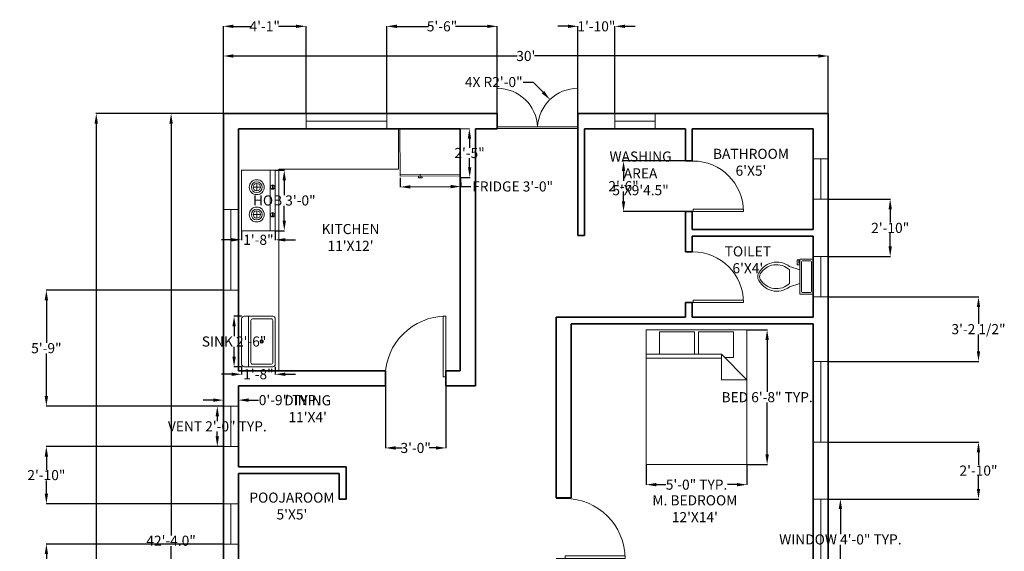
# Model space of a CAD drawing. Units: inches. Extents: x 94 to 277359, y -289541 to 1081.
# Tile 3 of 5: x 94 to 680, y 765 to 1081. Entities that reach past the tile are written whole.
import ezdxf

# ---------------------------------------------------------------- set-up
doc = ezdxf.new("R2010")
doc.units = ezdxf.units.IN
doc.header["$MEASUREMENT"] = 0
doc.layers.get('Defpoints').update_dxf_attribs({"color": 255})
for name, color, linetype, lineweight in [('A-ANNO-DIMS', 2, 'Continuous', 18), ('A-AREA-IDEN', 7, 'Continuous', 18), ('A-DOOR', 4, 'Continuous', 18), ('A-EQPM', 8, 'Continuous', 18), ('A-FLOR-CASE', 8, 'Continuous', 18), ('A-FLOR-FIXT', 8, 'Continuous', 18), ('A-WALL', 7, 'Continuous', 35), ('furniture', 163, 'Continuous', 18), ('window', 13, 'Continuous', 18)]:
    doc.layers.add(name, color=color, linetype=linetype, lineweight=lineweight)
doc.styles.get("Standard").update_dxf_attribs({"font": 'arial.ttf'})
doc.dimstyles.get("Standard").update_dxf_attribs({"dimtxt": 6, "dimasz": 6, "dimexe": 0.18, "dimexo": 0.0625, "dimgap": 0.09, "dimtad": 0, "dimtih": 1, "dimtoh": 1, "dimdec": 1, "dimzin": 0, "dimdsep": 46, "dimlunit": 3, "dimtxsty": 'Standard', "dimcen": 0.09, "dimadec": 0, "dimazin": 0, "dimtfac": 1, "dimtdec": 1, "dimtofl": 0, "dimtmove": 0, "dimatfit": 3, "dimfxl": 1, "dimtolj": 1, "dimtzin": 0, "dimarcsym": 0})

# ---------------------------------------------------------------- blocks, each defined once
blk = doc.blocks.new('DOOR')
for p, q in [((-94.95, 365.26), (-85.95, 365.26)), ((-94.95, 317.26), (-94.95, 365.26)), ((-90.45, 365.26), (-90.45, 317.26)), ((-85.95, 365.26), (-85.95, 317.26)), ((-85.95, 317.26), (-94.95, 317.26))]:
    blk.add_line(p, q)
blk = doc.blocks.new('V')
for p, q in [((-17.52, 401.92), (-8.52, 401.92)), ((-17.52, 377.92), (-17.52, 401.92)), ((-13.02, 377.92), (-13.02, 401.92)), ((-8.52, 401.92), (-8.52, 377.92)), ((-8.52, 377.92), (-17.52, 377.92))]:
    blk.add_line(p, q)
blk = doc.blocks.new('*D3')
at = {"layer": 'A-ANNO-DIMS', "color": 0, "lineweight": -2, "transparency": 16777216}
for p, q in [((215.5, 1025.45), (139.73, 1025.45)), ((139.91, 1019.45), (139.91, 717.61)), ((139.91, 409.45), (139.91, 711.3)), ((215.5, 403.45), (139.73, 403.45))]:
    blk.add_line(p, q, dxfattribs=at)
at = {"layer": 'A-ANNO-DIMS', "color": 0, "transparency": 16777216}
for points in [[(138.91, 1019.45), (140.91, 1019.45), (139.91, 1025.45)], [(138.91, 409.45), (140.91, 409.45), (139.91, 403.45)]]:
    blk.add_solid(points, dxfattribs=at)
at = {"layer": 'Defpoints', "color": 0, "transparency": 16777216}
for p in [(139.91, 1025.45), (215.56, 1025.45), (215.56, 403.45)]:
    blk.add_point(p, dxfattribs=at)
at = {"layer": 'A-ANNO-DIMS', "color": 0, "transparency": 16777216, "insert": (139.91, 714.45), "char_height": 6, "attachment_point": 5}
blk.add_mtext('\\A1;51\'-10.0"', dxfattribs=at)
blk = doc.blocks.new('*D4')
at = {"layer": 'A-ANNO-DIMS', "color": 0, "lineweight": -2, "transparency": 16777216}
for p, q in [((215.5, 1025.45), (184.27, 1025.45)), ((184.45, 1019.45), (184.45, 774.61)), ((184.45, 523.45), (184.45, 768.3)), ((215.5, 517.45), (184.27, 517.45))]:
    blk.add_line(p, q, dxfattribs=at)
at = {"layer": 'A-ANNO-DIMS', "color": 0, "transparency": 16777216}
for points in [[(183.45, 1019.45), (185.45, 1019.45), (184.45, 1025.45)], [(183.45, 523.45), (185.45, 523.45), (184.45, 517.45)]]:
    blk.add_solid(points, dxfattribs=at)
at = {"layer": 'Defpoints', "color": 0, "transparency": 16777216}
for p in [(215.56, 1025.45), (184.45, 517.45), (215.56, 517.45)]:
    blk.add_point(p, dxfattribs=at)
at = {"layer": 'A-ANNO-DIMS', "color": 0, "transparency": 16777216, "insert": (184.45, 771.45), "char_height": 6, "attachment_point": 5}
blk.add_mtext('\\A1;42\'-4.0"', dxfattribs=at)
blk = doc.blocks.new('Bed - Queen')
for p, q in [((0, -80.00003), (0, 0)), ((0, 0), (59.99999, 0)), ((59.99999, 0), (59.99999, -80.00003)), ((7.99999, -1.2), (28.79998, -1.2)), ((7.99999, -14.4), (7.99999, -1.2)), ((28.79998, -1.2), (28.79998, -14.4)), ((31.19999, -1.2), (51.99999, -1.2)), ((31.19999, -14.4), (31.19999, -1.2)), ((51.99999, -1.2), (51.99999, -16.4)), ((0, -14.4), (44.8, -14.4)), ((44.8, -16.8), (0, -16.8)), ((59.99999, -29.6), (44.8, -14.4)), ((44.8, -14.4), (44.8, -29.6)), ((51.99999, -16.4), (46.79936, -16.4)), ((44.8, -29.6), (59.99999, -29.6)), ((59.99999, -80.00003), (0, -80.00003))]:
    blk.add_line(p, q)
blk = doc.blocks.new('Sink-single - 30 in top')
blk.add_line((-15, -3.999996), (15, -3.999996))
for points in [[(-13.5, 0), (13.5, 0)], [(-15, -18.499996), (-15, -1.5)], [(-12.5, -5.499996), (12.5, -5.499996)], [(15, -1.5), (15, -18.499996)], [(-13.5, -17.499996), (-13.5, -6.499996)], [(13.5, -6.499996), (13.5, -17.499996)], [(13.5, -19.999996), (-13.5, -19.999996)], [(12.5, -18.499996), (-12.5, -18.499996)]]:
    blk.add_lwpolyline(points)
for radius in [1, 0.5]:
    blk.add_circle((0, -11.999996), radius)
for centre, radius, start, end in [((-13.5, -1.5), 1.5, 90, 180), ((-12.5, -6.499996), 1, 90, 180), ((12.5, -6.499996), 1, 0, 90), ((13.5, -1.5), 1.5, 0, 90), ((-12.5, -17.499996), 1, 180, 270), ((12.5, -17.499996), 1, 270, 0), ((-13.5, -18.499996), 1.5, 180, 270), ((13.5, -18.499996), 1.5, 270, 0)]:
    blk.add_arc(centre, radius, start, end)
blk = doc.blocks.new('gas')
at = {"layer": 'furniture'}
for p, q in [((194.36, 516.15), (214.36, 516.15)), ((194.36, 480.15), (194.36, 516.15)), ((211.36, 516.15), (211.36, 480.15)), ((214.36, 516.15), (214.36, 480.15)), ((201.2, 506.04), (205.6, 506.04)), ((203.4, 503.83), (203.4, 508.24)), ((212.69, 504.83), (212.69, 507.37)), ((213.08, 504.83), (213.08, 507.37)), ((201.2, 489.79), (205.6, 489.79)), ((203.4, 487.59), (203.4, 492)), ((212.69, 488.4), (212.69, 490.95)), ((213.08, 488.4), (213.08, 490.94)), ((214.36, 480.15), (194.36, 480.15))]:
    blk.add_line(p, q, dxfattribs=at)
for centre, radius in [((203.4, 506.04), 4.44), ((203.4, 506.04), 3.22), ((203.4, 506.04), 2.2), ((212.86, 506.1), 1.29), ((203.4, 489.79), 4.44), ((203.4, 489.79), 3.22), ((203.4, 489.79), 2.2), ((212.86, 489.67), 1.29)]:
    blk.add_circle(centre, radius, dxfattribs=at)
blk = doc.blocks.new('Refrigerator-2 door - 36 in top')
for p, q in [((0, -26.999999), (36, -26.999999)), ((11, -27.999999), (11, -28.999999)), ((11, -28.999999), (13, -28.999999)), ((12, -26.999999), (12, -28.999999)), ((13, -28.999999), (13, -27.999999))]:
    blk.add_line(p, q)
blk.add_lwpolyline([(0, -27.999999), (0, 0), (36, 0), (36, -27.999999)], close=True)
blk = doc.blocks.new('Toilet - top')
for p, q in [((9.5, -6), (9.5, -2)), ((-10, -8.5), (-8, -8.5)), ((-10, -9.5), (-10, -8.5)), ((-7, -9.5), (-10, -9.5)), ((-8, -8.5), (-8, -8)), ((-7, -8), (-7, -9.5)), ((-4, -8), (-6, -14)), ((4, -8), (6, -14)), ((4, -14), (-4, -14))]:
    blk.add_line(p, q)
blk.add_lwpolyline([(10.5, -8), (10.5, 0), (-10.5, 0), (-10.5, -8)], close=True)
for points in [[(-9.5, -2), (-9.5, -6)], [(8.5, -1), (-8.5, -1)], [(-8.5, -7), (8.5, -7)]]:
    blk.add_lwpolyline(points)
for centre, radius, start, end in [((-8.62, -1.88), 0.884, 81.8699, 188.1301), ((8.62, -1.88), 0.884, 351.8699, 98.1301), ((-8.62, -6.12), 0.884, 171.8699, 278.1301), ((8.62, -6.12), 0.884, 261.8699, 8.1301), ((3.52, -21.58), 12.17, 141.46911, 247.97143), ((4.2, -21.82), 11.33, 136.36773, 238.94682), ((-3.52, -21.58), 12.17, 292.02843, 38.53071), ((-4.2, -21.82), 11.33, 301.05301, 43.63209), ((0, -27.88), 4, 245.73182, 294.26817), ((0, -29), 4, 254.86053, 285.13947)]:
    blk.add_arc(centre, radius, start, end)
blk = doc.blocks.new('MD')
for p, q in [((202.8, 674.18), (202.8, 698.18)), ((250.8, 674.18), (250.8, 698.18)), ((202.8, 675.18), (250.8, 675.18)), ((202.8, 674.18), (250.8, 674.18))]:
    blk.add_line(p, q)
for centre, start, end in [((202.8, 674.18), 2.38802, 90), ((250.8, 674.18), 90, 177.61198)]:
    blk.add_arc(centre, 24, start, end)
blk = doc.blocks.new('*U15')
for p, q in [((0, 0), (0, -6)), ((40, 0), (40, -6))]:
    blk.add_line(p, q)
blk.add_lwpolyline([(0, 0), (0, 40), (1.75, 40), (1.75, 0)], close=True)
blk.add_arc((0, 0), 40, 0, 90)
blk = doc.blocks.new('*D16')
at = {"layer": 'A-ANNO-DIMS', "color": 0, "lineweight": -2, "transparency": 16777216}
for p, q in [((215.56, 1025.52), (215.56, 1059.85)), ((221.56, 1059.67), (390.38, 1059.67)), ((569.56, 1059.67), (400.74, 1059.67)), ((575.56, 1025.52), (575.56, 1059.85))]:
    blk.add_line(p, q, dxfattribs=at)
at = {"layer": 'A-ANNO-DIMS', "color": 0, "transparency": 16777216}
for points in [[(221.56, 1060.67), (221.56, 1058.67), (215.56, 1059.67)], [(569.56, 1060.67), (569.56, 1058.67), (575.56, 1059.67)]]:
    blk.add_solid(points, dxfattribs=at)
at = {"layer": 'Defpoints', "color": 0, "transparency": 16777216}
for p in [(575.56, 1059.67), (215.56, 1025.45), (575.56, 1025.45)]:
    blk.add_point(p, dxfattribs=at)
at = {"layer": 'A-ANNO-DIMS', "color": 0, "transparency": 16777216, "insert": (395.56, 1059.67), "char_height": 6, "attachment_point": 5}
blk.add_mtext("\\A1;30'", dxfattribs=at)
blk = doc.blocks.new('*D21')
at = {"layer": 'A-ANNO-DIMS', "color": 0, "lineweight": -2, "transparency": 16777216}
for p, q in [((575.63, 796.21), (582.94, 796.21)), ((582.76, 790.21), (582.76, 775.41)), ((582.76, 754.21), (582.76, 769.02)), ((575.63, 748.21), (582.94, 748.21))]:
    blk.add_line(p, q, dxfattribs=at)
at = {"layer": 'A-ANNO-DIMS', "color": 0, "transparency": 16777216}
for points in [[(581.76, 790.21), (583.76, 790.21), (582.76, 796.21)], [(581.76, 754.21), (583.76, 754.21), (582.76, 748.21)]]:
    blk.add_solid(points, dxfattribs=at)
at = {"layer": 'Defpoints', "color": 0, "transparency": 16777216}
for p in [(575.56, 796.21), (582.76, 796.21), (575.56, 748.21)]:
    blk.add_point(p, dxfattribs=at)
at = {"layer": 'A-ANNO-DIMS', "color": 0, "transparency": 16777216, "insert": (582.76, 772.21), "char_height": 6, "attachment_point": 5}
blk.add_mtext('\\A1;WINDOW 4\'-0" TYP.', dxfattribs=at)
blk = doc.blocks.new('*D23')
at = {"layer": 'A-ANNO-DIMS', "color": 0, "lineweight": -2, "transparency": 16777216}
for p, q in [((215.5, 851.45), (211.78, 851.45)), ((211.96, 845.45), (211.96, 842.61)), ((211.96, 833.45), (211.96, 836.3)), ((215.5, 827.45), (211.78, 827.45))]:
    blk.add_line(p, q, dxfattribs=at)
at = {"layer": 'A-ANNO-DIMS', "color": 0, "transparency": 16777216}
for points in [[(210.96, 845.45), (212.96, 845.45), (211.96, 851.45)], [(210.96, 833.45), (212.96, 833.45), (211.96, 827.45)]]:
    blk.add_solid(points, dxfattribs=at)
at = {"layer": 'Defpoints', "color": 0, "transparency": 16777216}
for p in [(211.96, 851.45), (215.56, 851.45), (215.56, 827.45)]:
    blk.add_point(p, dxfattribs=at)
at = {"layer": 'A-ANNO-DIMS', "color": 0, "transparency": 16777216, "insert": (211.96, 839.45), "char_height": 6, "attachment_point": 5}
blk.add_mtext('\\A1;VENT 2\'-0" TYP.', dxfattribs=at)
blk = doc.blocks.new('*D24')
at = {"layer": 'A-ANNO-DIMS', "color": 0, "lineweight": -2, "transparency": 16777216}
for p, q in [((209.56, 855.05), (203.56, 855.05)), ((215.56, 851.52), (215.56, 855.23)), ((224.56, 851.52), (224.56, 855.23)), ((230.56, 855.05), (236.56, 855.05))]:
    blk.add_line(p, q, dxfattribs=at)
at = {"layer": 'A-ANNO-DIMS', "color": 0, "transparency": 16777216}
for points in [[(209.56, 856.05), (209.56, 854.05), (215.56, 855.05)], [(230.56, 856.05), (230.56, 854.05), (224.56, 855.05)]]:
    blk.add_solid(points, dxfattribs=at)
at = {"layer": 'Defpoints', "color": 0, "transparency": 16777216}
for p in [(215.56, 851.45), (224.56, 855.05), (224.56, 851.45)]:
    blk.add_point(p, dxfattribs=at)
at = {"layer": 'A-ANNO-DIMS', "color": 0, "transparency": 16777216, "insert": (254.94, 855.05), "char_height": 6, "attachment_point": 5}
blk.add_mtext('\\A1;0\'-9" TYP.', dxfattribs=at)
blk = doc.blocks.new('*D27')
at = {"layer": 'A-ANNO-DIMS', "color": 0, "lineweight": -2, "transparency": 16777216}
for p, q in [((527.23, 896.78), (539.35, 896.78)), ((539.17, 890.78), (539.17, 859.93)), ((539.17, 822.78), (539.17, 853.62)), ((527.23, 816.78), (539.35, 816.78))]:
    blk.add_line(p, q, dxfattribs=at)
at = {"layer": 'A-ANNO-DIMS', "color": 0, "transparency": 16777216}
for points in [[(538.17, 890.78), (540.17, 890.78), (539.17, 896.78)], [(538.17, 822.78), (540.17, 822.78), (539.17, 816.78)]]:
    blk.add_solid(points, dxfattribs=at)
at = {"layer": 'Defpoints', "color": 0, "transparency": 16777216}
for p in [(527.17, 896.78), (539.17, 896.78), (527.17, 816.78)]:
    blk.add_point(p, dxfattribs=at)
at = {"layer": 'A-ANNO-DIMS', "color": 0, "transparency": 16777216, "insert": (539.17, 856.78), "char_height": 6, "attachment_point": 5}
blk.add_mtext('\\A1;BED 6\'-8" TYP.', dxfattribs=at)
blk = doc.blocks.new('*D28')
at = {"layer": 'A-ANNO-DIMS', "color": 0, "lineweight": -2, "transparency": 16777216}
for p, q in [((467.17, 816.71), (467.17, 804.6)), ((527.17, 816.71), (527.17, 804.6)), ((473.17, 804.78), (478.79, 804.78)), ((521.17, 804.78), (515.54, 804.78))]:
    blk.add_line(p, q, dxfattribs=at)
at = {"layer": 'A-ANNO-DIMS', "color": 0, "transparency": 16777216}
for points in [[(473.17, 805.78), (473.17, 803.78), (467.17, 804.78)], [(521.17, 805.78), (521.17, 803.78), (527.17, 804.78)]]:
    blk.add_solid(points, dxfattribs=at)
at = {"layer": 'Defpoints', "color": 0, "transparency": 16777216}
for p in [(467.17, 816.78), (527.17, 816.78), (527.17, 804.78)]:
    blk.add_point(p, dxfattribs=at)
at = {"layer": 'A-ANNO-DIMS', "color": 0, "transparency": 16777216, "insert": (497.17, 804.78), "char_height": 6, "attachment_point": 5}
blk.add_mtext('\\A1;5\'-0" TYP.', dxfattribs=at)
blk = doc.blocks.new('*D39')
at = {"layer": 'A-ANNO-DIMS', "color": 0, "lineweight": -2, "transparency": 16777216}
for p, q in [((226.37, 904.91), (221.76, 904.91)), ((221.94, 898.91), (221.94, 893.1)), ((221.94, 880.91), (221.94, 886.71)), ((226.37, 874.91), (221.76, 874.91))]:
    blk.add_line(p, q, dxfattribs=at)
at = {"layer": 'A-ANNO-DIMS', "color": 0, "transparency": 16777216}
for points in [[(220.94, 898.91), (222.94, 898.91), (221.94, 904.91)], [(220.94, 880.91), (222.94, 880.91), (221.94, 874.91)]]:
    blk.add_solid(points, dxfattribs=at)
at = {"layer": 'Defpoints', "color": 0, "transparency": 16777216}
for p in [(221.94, 904.91), (226.44, 904.91), (226.44, 874.91)]:
    blk.add_point(p, dxfattribs=at)
at = {"layer": 'A-ANNO-DIMS', "color": 0, "transparency": 16777216, "insert": (221.94, 889.91), "char_height": 6, "attachment_point": 5}
blk.add_mtext('\\A1;SINK 2\'-6"', dxfattribs=at)
blk = doc.blocks.new('*D40')
at = {"layer": 'A-ANNO-DIMS', "color": 0, "lineweight": -2, "transparency": 16777216}
for p, q in [((226.44, 874.84), (226.44, 870.23)), ((246.44, 874.84), (246.44, 870.23)), ((220.44, 870.41), (214.44, 870.41)), ((252.44, 870.41), (258.44, 870.41))]:
    blk.add_line(p, q, dxfattribs=at)
at = {"layer": 'A-ANNO-DIMS', "color": 0, "transparency": 16777216}
for points in [[(220.44, 871.41), (220.44, 869.41), (226.44, 870.41)], [(252.44, 871.41), (252.44, 869.41), (246.44, 870.41)]]:
    blk.add_solid(points, dxfattribs=at)
at = {"layer": 'Defpoints', "color": 0, "transparency": 16777216}
for p in [(226.44, 874.91), (246.44, 874.91), (226.44, 870.41)]:
    blk.add_point(p, dxfattribs=at)
at = {"layer": 'A-ANNO-DIMS', "color": 0, "transparency": 16777216, "insert": (236.44, 870.41), "char_height": 6, "attachment_point": 5}
blk.add_mtext('\\A1;1\'-8"', dxfattribs=at)
blk = doc.blocks.new('*D41')
at = {"layer": 'A-ANNO-DIMS', "color": 0, "lineweight": -2, "transparency": 16777216}
for p, q in [((246.46, 991.77), (251.98, 991.77)), ((251.8, 985.77), (251.8, 976.97)), ((251.8, 961.77), (251.8, 970.58)), ((246.46, 955.77), (251.98, 955.77))]:
    blk.add_line(p, q, dxfattribs=at)
at = {"layer": 'A-ANNO-DIMS', "color": 0, "transparency": 16777216}
for points in [[(250.8, 985.77), (252.8, 985.77), (251.8, 991.77)], [(250.8, 961.77), (252.8, 961.77), (251.8, 955.77)]]:
    blk.add_solid(points, dxfattribs=at)
at = {"layer": 'Defpoints', "color": 0, "transparency": 16777216}
for p in [(246.4, 991.77), (251.8, 991.77), (246.4, 955.77)]:
    blk.add_point(p, dxfattribs=at)
at = {"layer": 'A-ANNO-DIMS', "color": 0, "transparency": 16777216, "insert": (251.8, 973.77), "char_height": 6, "attachment_point": 5}
blk.add_mtext('\\A1;HOB 3\'-0"', dxfattribs=at)
blk = doc.blocks.new('*D42')
at = {"layer": 'A-ANNO-DIMS', "color": 0, "lineweight": -2, "transparency": 16777216}
for p, q in [((226.4, 955.71), (226.4, 950.19)), ((246.4, 955.71), (246.4, 950.19)), ((220.4, 950.37), (214.4, 950.37)), ((252.4, 950.37), (258.4, 950.37))]:
    blk.add_line(p, q, dxfattribs=at)
at = {"layer": 'A-ANNO-DIMS', "color": 0, "transparency": 16777216}
for points in [[(220.4, 951.37), (220.4, 949.37), (226.4, 950.37)], [(252.4, 951.37), (252.4, 949.37), (246.4, 950.37)]]:
    blk.add_solid(points, dxfattribs=at)
at = {"layer": 'Defpoints', "color": 0, "transparency": 16777216}
for p in [(226.4, 955.77), (246.4, 955.77), (246.4, 950.37)]:
    blk.add_point(p, dxfattribs=at)
at = {"layer": 'A-ANNO-DIMS', "color": 0, "transparency": 16777216, "insert": (236.4, 950.37), "char_height": 6, "attachment_point": 5}
blk.add_mtext('\\A1;1\'-8"', dxfattribs=at)
blk = doc.blocks.new('*D43')
at = {"layer": 'A-ANNO-DIMS', "color": 0, "lineweight": -2, "transparency": 16777216}
for p, q in [((320.78, 987.12), (320.83, 981.6)), ((356.78, 987.39), (356.83, 981.87)), ((326.82, 981.83), (350.82, 982.01)), ((356.82, 982.05), (362.82, 982.1))]:
    blk.add_line(p, q, dxfattribs=at)
at = {"layer": 'A-ANNO-DIMS', "color": 0, "transparency": 16777216}
for points in [[(326.82, 982.83), (326.83, 980.83), (320.82, 981.78)], [(350.82, 983.01), (350.83, 981.01), (356.82, 982.05)]]:
    blk.add_solid(points, dxfattribs=at)
at = {"layer": 'Defpoints', "color": 0, "transparency": 16777216}
for p in [(320.78, 987.18), (356.78, 987.45), (356.82, 982.05)]:
    blk.add_point(p, dxfattribs=at)
at = {"layer": 'A-ANNO-DIMS', "color": 0, "transparency": 16777216, "insert": (387.72, 982.1), "char_height": 6, "attachment_point": 5}
blk.add_mtext('\\A1;FRIDGE 3\'-0"', dxfattribs=at)
blk = doc.blocks.new('*D44')
at = {"layer": 'A-ANNO-DIMS', "color": 0, "lineweight": -2, "transparency": 16777216}
for p, q in [((356.63, 1016.45), (362.14, 1016.5)), ((362.01, 1010.49), (362.05, 1005.15)), ((362.14, 993.5), (362.1, 998.84)), ((356.85, 987.45), (362.36, 987.5))]:
    blk.add_line(p, q, dxfattribs=at)
at = {"layer": 'A-ANNO-DIMS', "color": 0, "transparency": 16777216}
for points in [[(363.01, 1010.5), (361.01, 1010.49), (361.96, 1016.49)], [(363.14, 993.5), (361.14, 993.49), (362.18, 987.5)]]:
    blk.add_solid(points, dxfattribs=at)
at = {"layer": 'Defpoints', "color": 0, "transparency": 16777216}
for p in [(356.56, 1016.45), (361.96, 1016.49), (356.78, 987.45)]:
    blk.add_point(p, dxfattribs=at)
at = {"layer": 'A-ANNO-DIMS', "color": 0, "transparency": 16777216, "insert": (362.07, 1001.99), "char_height": 6, "attachment_point": 5}
blk.add_mtext('\\A1;2\'-5"', dxfattribs=at)
blk = doc.blocks.new('*D49')
at = {"layer": 'A-ANNO-DIMS', "color": 0, "lineweight": -2, "transparency": 16777216}
for p, q in [((215.56, 1025.52), (215.56, 1077.48)), ((221.56, 1077.3), (232, 1077.3)), ((258.8, 1077.3), (248.37, 1077.3)), ((264.8, 1025.52), (264.8, 1077.48))]:
    blk.add_line(p, q, dxfattribs=at)
at = {"layer": 'A-ANNO-DIMS', "color": 0, "transparency": 16777216}
for points in [[(221.56, 1078.3), (221.56, 1076.3), (215.56, 1077.3)], [(258.8, 1078.3), (258.8, 1076.3), (264.8, 1077.3)]]:
    blk.add_solid(points, dxfattribs=at)
at = {"layer": 'Defpoints', "color": 0, "transparency": 16777216}
for p in [(264.8, 1077.3), (215.56, 1025.45), (264.8, 1025.45)]:
    blk.add_point(p, dxfattribs=at)
at = {"layer": 'A-ANNO-DIMS', "color": 0, "transparency": 16777216, "insert": (240.18, 1077.3), "char_height": 6, "attachment_point": 5}
blk.add_mtext('\\A1;4\'-1"', dxfattribs=at)
blk = doc.blocks.new('*D50')
at = {"layer": 'A-ANNO-DIMS', "color": 0, "lineweight": -2, "transparency": 16777216}
for p, q in [((312.8, 1025.52), (312.8, 1077.48)), ((318.8, 1077.3), (337.62, 1077.3)), ((372.56, 1077.3), (353.75, 1077.3)), ((378.56, 1025.52), (378.56, 1077.48))]:
    blk.add_line(p, q, dxfattribs=at)
at = {"layer": 'A-ANNO-DIMS', "color": 0, "transparency": 16777216}
for points in [[(318.8, 1078.3), (318.8, 1076.3), (312.8, 1077.3)], [(372.56, 1078.3), (372.56, 1076.3), (378.56, 1077.3)]]:
    blk.add_solid(points, dxfattribs=at)
at = {"layer": 'Defpoints', "color": 0, "transparency": 16777216}
for p in [(378.56, 1077.3), (312.8, 1025.45), (378.56, 1025.45)]:
    blk.add_point(p, dxfattribs=at)
at = {"layer": 'A-ANNO-DIMS', "color": 0, "transparency": 16777216, "insert": (345.68, 1077.3), "char_height": 6, "attachment_point": 5}
blk.add_mtext('\\A1;5\'-6"', dxfattribs=at)
blk = doc.blocks.new('*D51')
at = {"layer": 'A-ANNO-DIMS', "color": 0, "lineweight": -2, "transparency": 16777216}
for p, q in [((420.562785, 1077.303348), (414.562785, 1077.303348)), ((426.562785, 1025.515848), (426.562785, 1077.483348)), ((448.562785, 1025.515848), (448.562785, 1077.483348)), ((454.562785, 1077.303348), (460.562785, 1077.303348))]:
    blk.add_line(p, q, dxfattribs=at)
at = {"layer": 'A-ANNO-DIMS', "color": 0, "transparency": 16777216}
for points in [[(420.562785, 1078.303348), (420.562785, 1076.303348), (426.562785, 1077.303348)], [(454.562785, 1078.303348), (454.562785, 1076.303348), (448.562785, 1077.303348)]]:
    blk.add_solid(points, dxfattribs=at)
at = {"layer": 'Defpoints', "color": 0, "transparency": 16777216}
for p in [(448.562785, 1077.303348), (426.562785, 1025.453348), (448.562785, 1025.453348)]:
    blk.add_point(p, dxfattribs=at)
at = {"layer": 'A-ANNO-DIMS', "color": 0, "transparency": 16777216, "insert": (437.562785, 1077.303348), "char_height": 6, "attachment_point": 5}
blk.add_mtext('\\A1;1\'-10"', dxfattribs=at)
blk = doc.blocks.new('*D52')
at = {"layer": 'A-ANNO-DIMS', "color": 0, "lineweight": -2, "transparency": 16777216}
for p, q in [((312.01, 863.39), (312.01, 826.42)), ((348.01, 863.39), (348.01, 826.42)), ((318.01, 826.6), (321.95, 826.6)), ((342.01, 826.6), (338.08, 826.6))]:
    blk.add_line(p, q, dxfattribs=at)
at = {"layer": 'A-ANNO-DIMS', "color": 0, "transparency": 16777216}
for points in [[(318.01, 827.6), (318.01, 825.6), (312.01, 826.6)], [(342.01, 827.6), (342.01, 825.6), (348.01, 826.6)]]:
    blk.add_solid(points, dxfattribs=at)
at = {"layer": 'Defpoints', "color": 0, "transparency": 16777216}
for p in [(312.01, 863.45), (348.01, 863.45), (312.01, 826.6)]:
    blk.add_point(p, dxfattribs=at)
at = {"layer": 'A-ANNO-DIMS', "color": 0, "transparency": 16777216, "insert": (330.01, 826.6), "char_height": 6, "attachment_point": 5}
blk.add_mtext('\\A1;3\'-0"', dxfattribs=at)
blk = doc.blocks.new('*D53')
at = {"layer": 'A-ANNO-DIMS', "color": 0, "lineweight": -2, "transparency": 16777216}
for p, q in [((490.5, 997.24), (453.53, 997.24)), ((453.71, 991.24), (453.71, 985.39)), ((453.71, 973.24), (453.71, 979.08)), ((490.5, 967.24), (453.53, 967.24))]:
    blk.add_line(p, q, dxfattribs=at)
at = {"layer": 'A-ANNO-DIMS', "color": 0, "transparency": 16777216}
for points in [[(452.71, 991.24), (454.71, 991.24), (453.71, 997.24)], [(452.71, 973.24), (454.71, 973.24), (453.71, 967.24)]]:
    blk.add_solid(points, dxfattribs=at)
at = {"layer": 'Defpoints', "color": 0, "transparency": 16777216}
for p in [(453.71, 997.24), (490.56, 997.24), (490.56, 967.24)]:
    blk.add_point(p, dxfattribs=at)
at = {"layer": 'A-ANNO-DIMS', "color": 0, "transparency": 16777216, "insert": (453.71, 982.24), "char_height": 6, "attachment_point": 5}
blk.add_mtext('\\A1;2\'-6"', dxfattribs=at)
blk = doc.blocks.new('*D56')
at = {"layer": 'A-ANNO-DIMS', "color": 0, "lineweight": -2, "transparency": 16777216}
for p, q in [((215.5, 769.45), (110.05, 769.45)), ((110.23, 763.45), (110.23, 740.35)), ((110.23, 710.86), (110.23, 733.96)), ((215.5, 704.86), (110.05, 704.86))]:
    blk.add_line(p, q, dxfattribs=at)
at = {"layer": 'A-ANNO-DIMS', "color": 0, "transparency": 16777216}
for points in [[(109.23, 763.45), (111.23, 763.45), (110.23, 769.45)], [(109.23, 710.86), (111.23, 710.86), (110.23, 704.86)]]:
    blk.add_solid(points, dxfattribs=at)
at = {"layer": 'Defpoints', "color": 0, "transparency": 16777216}
for p in [(110.23, 769.45), (215.56, 769.45), (215.56, 704.86)]:
    blk.add_point(p, dxfattribs=at)
at = {"layer": 'A-ANNO-DIMS', "color": 0, "transparency": 16777216, "insert": (110.23, 737.16), "char_height": 6, "attachment_point": 5}
blk.add_mtext('\\A1;5\'-4 1/2"', dxfattribs=at)
blk = doc.blocks.new('*D57')
at = {"layer": 'A-ANNO-DIMS', "color": 0, "lineweight": -2, "transparency": 16777216}
for p, q in [((215.5, 827.45), (110.05, 827.45)), ((110.23, 821.45), (110.23, 813.61)), ((110.23, 799.45), (110.23, 807.3)), ((215.5, 793.45), (110.05, 793.45))]:
    blk.add_line(p, q, dxfattribs=at)
at = {"layer": 'A-ANNO-DIMS', "color": 0, "transparency": 16777216}
for points in [[(109.23, 821.45), (111.23, 821.45), (110.23, 827.45)], [(109.23, 799.45), (111.23, 799.45), (110.23, 793.45)]]:
    blk.add_solid(points, dxfattribs=at)
at = {"layer": 'Defpoints', "color": 0, "transparency": 16777216}
for p in [(110.23, 827.45), (215.56, 827.45), (215.56, 793.45)]:
    blk.add_point(p, dxfattribs=at)
at = {"layer": 'A-ANNO-DIMS', "color": 0, "transparency": 16777216, "insert": (110.23, 810.45), "char_height": 6, "attachment_point": 5}
blk.add_mtext('\\A1;2\'-10"', dxfattribs=at)
blk = doc.blocks.new('*D58')
at = {"layer": 'A-ANNO-DIMS', "color": 0, "lineweight": -2, "transparency": 16777216}
for p, q in [((215.5, 920.45), (110.05, 920.45)), ((110.23, 914.45), (110.23, 889.11)), ((110.23, 857.45), (110.23, 882.8)), ((215.5, 851.45), (110.05, 851.45))]:
    blk.add_line(p, q, dxfattribs=at)
at = {"layer": 'A-ANNO-DIMS', "color": 0, "transparency": 16777216}
for points in [[(109.23, 914.45), (111.23, 914.45), (110.23, 920.45)], [(109.23, 857.45), (111.23, 857.45), (110.23, 851.45)]]:
    blk.add_solid(points, dxfattribs=at)
at = {"layer": 'Defpoints', "color": 0, "transparency": 16777216}
for p in [(110.23, 920.45), (215.56, 920.45), (215.56, 851.45)]:
    blk.add_point(p, dxfattribs=at)
at = {"layer": 'A-ANNO-DIMS', "color": 0, "transparency": 16777216, "insert": (110.23, 885.95), "char_height": 6, "attachment_point": 5}
blk.add_mtext('\\A1;5\'-9"', dxfattribs=at)
blk = doc.blocks.new('*D62')
at = {"layer": 'A-ANNO-DIMS', "color": 0, "lineweight": -2, "transparency": 16777216}
for p, q in [((575.63, 830.05), (665.14, 830.05)), ((664.96, 824.05), (664.96, 816.28)), ((664.96, 802.21), (664.96, 809.98)), ((575.63, 796.21), (665.14, 796.21))]:
    blk.add_line(p, q, dxfattribs=at)
at = {"layer": 'A-ANNO-DIMS', "color": 0, "transparency": 16777216}
for points in [[(663.96, 824.05), (665.96, 824.05), (664.96, 830.05)], [(663.96, 802.21), (665.96, 802.21), (664.96, 796.21)]]:
    blk.add_solid(points, dxfattribs=at)
at = {"layer": 'Defpoints', "color": 0, "transparency": 16777216}
for p in [(575.56, 830.05), (575.56, 796.21), (664.96, 796.21)]:
    blk.add_point(p, dxfattribs=at)
at = {"layer": 'A-ANNO-DIMS', "color": 0, "transparency": 16777216, "insert": (664.96, 813.13), "char_height": 6, "attachment_point": 5}
blk.add_mtext('\\A1;2\'-10"', dxfattribs=at)
blk = doc.blocks.new('*D63')
at = {"layer": 'A-ANNO-DIMS', "color": 0, "lineweight": -2, "transparency": 16777216}
for p, q in [((575.63, 916.45), (665.14, 916.45)), ((664.96, 910.45), (664.96, 900.44)), ((664.96, 884.05), (664.96, 894.06)), ((575.63, 878.05), (665.14, 878.05))]:
    blk.add_line(p, q, dxfattribs=at)
at = {"layer": 'A-ANNO-DIMS', "color": 0, "transparency": 16777216}
for points in [[(663.96, 910.45), (665.96, 910.45), (664.96, 916.45)], [(663.96, 884.05), (665.96, 884.05), (664.96, 878.05)]]:
    blk.add_solid(points, dxfattribs=at)
at = {"layer": 'Defpoints', "color": 0, "transparency": 16777216}
for p in [(575.56, 916.45), (575.56, 878.05), (664.96, 878.05)]:
    blk.add_point(p, dxfattribs=at)
at = {"layer": 'A-ANNO-DIMS', "color": 0, "transparency": 16777216, "insert": (664.96, 897.25), "char_height": 6, "attachment_point": 5}
blk.add_mtext('\\A1;3\'-2 1/2"', dxfattribs=at)
blk = doc.blocks.new('*D64')
at = {"layer": 'A-ANNO-DIMS', "color": 0, "lineweight": -2, "transparency": 16777216}
for p, q in [((575.63, 974.45), (612.59, 974.45)), ((612.41, 968.45), (612.41, 960.61)), ((612.41, 946.45), (612.41, 954.3)), ((575.63, 940.45), (612.59, 940.45))]:
    blk.add_line(p, q, dxfattribs=at)
at = {"layer": 'A-ANNO-DIMS', "color": 0, "transparency": 16777216}
for points in [[(611.41, 968.45), (613.41, 968.45), (612.41, 974.45)], [(611.41, 946.45), (613.41, 946.45), (612.41, 940.45)]]:
    blk.add_solid(points, dxfattribs=at)
at = {"layer": 'Defpoints', "color": 0, "transparency": 16777216}
for p in [(575.56, 974.45), (575.56, 940.45), (612.41, 940.45)]:
    blk.add_point(p, dxfattribs=at)
at = {"layer": 'A-ANNO-DIMS', "color": 0, "transparency": 16777216, "insert": (612.41, 957.45), "char_height": 6, "attachment_point": 5}
blk.add_mtext('\\A1;2\'-10"', dxfattribs=at)
blk = doc.blocks.new('*D96')
at = {"layer": 'A-ANNO-DIMS', "color": 0, "lineweight": -2, "transparency": 16777216}
for p, q in [((393.98, 1044.17), (399.98, 1044.17)), ((399.98, 1044.17), (405.8, 1038.1)), ((426.47, 1016.45), (426.65, 1016.45)), ((426.56, 1016.36), (426.56, 1016.54))]:
    blk.add_line(p, q, dxfattribs=at)
at = {"layer": 'A-ANNO-DIMS', "color": 0, "transparency": 16777216}
blk.add_solid([(406.52, 1038.8), (405.07, 1037.41), (409.95, 1033.77)], dxfattribs=at)
at = {"layer": 'Defpoints', "color": 0, "transparency": 16777216}
for p in [(409.95, 1033.77), (426.56, 1016.45)]:
    blk.add_point(p, dxfattribs=at)
at = {"layer": 'A-ANNO-DIMS', "color": 0, "transparency": 16777216, "insert": (376.48, 1044.17), "char_height": 6, "attachment_point": 5}
blk.add_mtext('\\A1;4X R2\'-0"', dxfattribs=at)

msp = doc.modelspace()

# ---------------------------------------------------------------- linework, layer by layer
at = {"layer": 'A-FLOR-CASE'}
for p, q in [((319.82, 992.45), (319.82, 1016.45)), ((319.82, 992.45), (248.56, 992.45)), ((248.56, 992.45), (248.56, 872.45))]:
    msp.add_line(p, q, dxfattribs=at)
at = {"layer": 'A-WALL'}
for p, q in [((215.56, 1025.45), (215.56, 403.45)), ((378.56, 1025.45), (215.56, 1025.45)), ((378.56, 1016.45), (378.56, 1025.45)), ((575.56, 1025.45), (426.56, 1025.45)), ((426.56, 1016.45), (426.56, 1025.45)), ((575.56, 403.45), (575.56, 1025.45)), ((224.56, 1016.45), (224.56, 872.45)), ((356.56, 1016.45), (224.56, 1016.45)), ((356.56, 1016.45), (356.56, 872.45)), ((365.56, 1016.45), (365.56, 863.45)), ((378.56, 1016.45), (365.56, 1016.45)), ((426.56, 952.9), (426.56, 1016.45)), ((490.56, 1016.45), (430.56, 1016.45)), ((430.56, 952.9), (430.56, 1016.45)), ((490.56, 997.24), (490.56, 1016.45)), ((566.56, 1016.45), (494.56, 1016.45)), ((494.56, 997.24), (494.56, 1016.45)), ((566.56, 956.45), (566.56, 1016.45)), ((494.56, 997.24), (490.56, 997.24)), ((490.56, 943.14), (490.56, 967.24)), ((494.56, 967.24), (490.56, 967.24)), ((494.56, 956.45), (494.56, 967.24)), ((566.56, 956.45), (494.56, 956.45)), ((426.56, 952.9), (430.56, 952.9)), ((566.56, 952.45), (494.56, 952.45)), ((494.56, 943.14), (494.56, 952.45)), ((566.56, 904.45), (566.56, 952.45)), ((490.56, 943.14), (494.56, 943.14)), ((490.56, 904.45), (490.56, 913.14)), ((490.56, 913.14), (494.56, 913.14)), ((494.56, 904.45), (494.56, 913.14)), ((490.56, 904.45), (413.56, 904.45)), ((413.56, 796.86), (413.56, 904.45)), ((566.56, 904.45), (494.56, 904.45)), ((566.56, 900.45), (422.56, 900.45)), ((422.56, 796.86), (422.56, 900.45)), ((566.56, 732.45), (566.56, 900.45)), ((312.01, 872.45), (224.56, 872.45)), ((312.01, 863.45), (312.01, 872.45)), ((356.56, 872.45), (348.01, 872.45)), ((348.01, 863.45), (348.01, 872.45)), ((224.56, 863.45), (224.56, 815.45)), ((312.01, 863.45), (224.56, 863.45)), ((365.56, 863.45), (348.01, 863.45)), ((288.56, 815.45), (224.56, 815.45)), ((288.56, 815.45), (288.56, 796.07)), ((284.56, 811.45), (224.56, 811.45)), ((224.56, 811.45), (224.56, 751.45)), ((284.56, 811.45), (284.56, 796.07)), ((284.56, 796.07), (288.56, 796.07)), ((413.56, 796.86), (422.56, 796.86))]:
    msp.add_line(p, q, dxfattribs=at)

# ---------------------------------------------------------------- block references
at = {"layer": 'A-DOOR'}
msp.add_blockref('MD', (175.76, 342.28), dxfattribs=at)
at = {"layer": 'A-DOOR', "rotation": 270}
for p, xscale, yscale, zscale in [((495.06, 967.24), -0.749682497870124, 0.749682497870124, 0.749682497870124), ((495.06, 913.14), -0.7502015302743262, 0.7502015302743262, 0.7502015302743262), ((418.92, 760.86), -0.8921197571226785, 0.8921197571226785, 0.8921197571226785)]:
    msp.add_blockref('*U15', p, dxfattribs=dict(at, xscale=xscale, yscale=yscale, zscale=zscale))
at = {"layer": 'A-DOOR', "xscale": -0.9015294236647445, "yscale": 0.9015294236647445, "zscale": 0.9015294236647445}
msp.add_blockref('*U15', (348.01, 868.86), dxfattribs=at)
at = {"layer": 'A-EQPM', "rotation": 0.4350136191508041}
msp.add_blockref('Refrigerator-2 door - 36 in top', (320.56, 1016.18), dxfattribs=at)
at = {"layer": 'A-EQPM'}
msp.add_blockref('gas', (32.04, 475.62), dxfattribs=at)
at = {"layer": 'A-FLOR-FIXT'}
for name, p, rotation in [('Toilet - top', (566.56, 928.45), 270), ('Sink-single - 30 in top', (226.44, 889.91), 89.99999999999999)]:
    msp.add_blockref(name, p, dxfattribs=dict(at, rotation=rotation))
at = {"layer": 'furniture'}
msp.add_blockref('Bed - Queen', (467.17, 896.78), dxfattribs=at)
at = {"layer": 'window', "rotation": 270}
for name, p in [('DOOR', (-52.45, 930.5)), ('V', (70.65, 1007.93))]:
    msp.add_blockref(name, p, dxfattribs=at)
at = {"layer": 'window'}
for name, p in [('V', (584.08, 596.54)), ('DOOR', (310.51, 603.2)), ('V', (584.08, 538.54)), ('DOOR', (661.51, 512.79)), ('V', (233.08, 449.54)), ('V', (233.08, 391.54)), ('DOOR', (661.51, 430.96))]:
    msp.add_blockref(name, p, dxfattribs=at)

# ---------------------------------------------------------------- texts
at = {"layer": 'A-AREA-IDEN', "char_height": 6, "attachment_point": 2}
for s, insert in [('WASHING\\PAREA\\P5\'X9\'4.5"', (463.84, 1002.88)), ("BATHROOM\\P6'X5'", (529.55, 1004.48)), ("KITCHEN\\P11'X12'", (291.24, 959.77)), ("TOILET\\P6'X4'", (527.69, 946.49)), ("DINING\\P11'X4'", (265.73, 857.93)), ("POOJAROOM\\P5'X5'", (256.37, 800.08)), ("M. BEDROOM\\P12'X14'", (496.17, 798.47))]:
    msp.add_mtext_dynamic_manual_height_columns(s, width=54.0436, gutter_width=1, heights=[0], dxfattribs=dict(at, insert=insert))

# ---------------------------------------------------------------- dimensions: what is measured, and where the dimension line sits
at = {"layer": 'A-ANNO-DIMS'}
for base, p1, p2, override, picture, middle in [((264.8, 1077.3), (215.56, 1025.45), (264.8, 1025.45), {"dimdec": 1, "dimlfac": 1, "dimrnd": 0, "dimzin": 1, "dimdsep": 46, "dimlunit": 4, "dimfrac": 2}, '*D49', (240.18, 1077.3)), ((378.56, 1077.3), (312.8, 1025.45), (378.56, 1025.45), {"dimdec": 1, "dimlfac": 1, "dimrnd": 0, "dimzin": 1, "dimdsep": 46, "dimlunit": 4, "dimfrac": 2}, '*D50', (345.68, 1077.3)), ((448.56, 1077.3), (426.56, 1025.45), (448.56, 1025.45), {"dimdec": 1, "dimlfac": 1, "dimrnd": 0, "dimzin": 1, "dimdsep": 46, "dimlunit": 4, "dimfrac": 2}, '*D51', (437.56, 1077.3)), ((575.56, 1059.67), (215.56, 1025.45), (575.56, 1025.45), {"dimclrd": 0, "dimclre": 0, "dimclrt": 0}, '*D16', (395.56, 1059.67)), ((246.4, 950.37), (226.4, 955.77), (246.4, 955.77), {"dimdec": 1, "dimlfac": 1, "dimrnd": 0, "dimzin": 1, "dimdsep": 46, "dimlunit": 4, "dimfrac": 2}, '*D42', (236.4, 950.37))]:
    dim = msp.add_linear_dim(base=base, p1=p1, p2=p2, dimstyle='Standard', override=override, dxfattribs=at)
    dim.commit()
    dim.dimension.update_dxf_attribs({"geometry": picture, "text_midpoint": middle})
dim = msp.add_radius_dim(center=(426.56, 1016.45), mpoint=(409.95, 1033.77), text='4X <>', dimstyle='Standard', override={"dimdec": 1, "dimlfac": 1, "dimrnd": 0, "dimzin": 1, "dimdsep": 46, "dimlunit": 4, "dimfrac": 2}, dxfattribs=at)
dim.commit()
dim.dimension.update_dxf_attribs({"geometry": '*D96', "text_midpoint": (376.48, 1044.17), "dimtype": 164})
for base, p1, p2, angle, override, picture, middle in [((139.91, 1025.45), (215.56, 403.45), (215.56, 1025.45), 90, {"dimclrd": 0, "dimclre": 0, "dimclrt": 0}, '*D3', (139.91, 714.45)), ((184.45, 517.45), (215.56, 1025.45), (215.56, 517.45), 90, {"dimclrd": 0, "dimclre": 0, "dimclrt": 0}, '*D4', (184.45, 771.45)), ((361.96, 1016.49), (356.78, 987.45), (356.56, 1016.45), 90.43501, {"dimdec": 1, "dimlfac": 1, "dimrnd": 0, "dimzin": 1, "dimdsep": 46, "dimlunit": 4, "dimfrac": 2}, '*D44', (362.07, 1001.99)), ((453.71, 997.24), (490.56, 967.24), (490.56, 997.24), 90, {"dimdec": 1, "dimlfac": 1, "dimrnd": 0, "dimzin": 1, "dimdsep": 46, "dimlunit": 4, "dimfrac": 2}, '*D53', (453.71, 982.24)), ((612.41, 940.45), (575.56, 974.45), (575.56, 940.45), 270, {"dimdec": 1, "dimlfac": 1, "dimrnd": 0, "dimzin": 1, "dimdsep": 46, "dimlunit": 4, "dimfrac": 2}, '*D64', (612.41, 957.45)), ((110.23, 920.45), (215.56, 851.45), (215.56, 920.45), 90, {"dimdec": 1, "dimlfac": 1, "dimrnd": 0, "dimzin": 1, "dimdsep": 46, "dimlunit": 4, "dimfrac": 2}, '*D58', (110.23, 885.95)), ((664.96, 878.05), (575.56, 916.45), (575.56, 878.05), 90, {"dimdec": 1, "dimlfac": 1, "dimrnd": 0, "dimzin": 1, "dimdsep": 46, "dimlunit": 4, "dimfrac": 2}, '*D63', (664.96, 897.25)), ((226.44, 870.41), (246.44, 874.91), (226.44, 874.91), 180, {"dimdec": 1, "dimlfac": 1, "dimrnd": 0, "dimzin": 1, "dimdsep": 46, "dimlunit": 4, "dimfrac": 2}, '*D40', (236.44, 870.41)), ((312.01, 826.6), (348.01, 863.45), (312.01, 863.45), 180, {"dimdec": 1, "dimlfac": 1, "dimrnd": 0, "dimzin": 1, "dimdsep": 46, "dimlunit": 4, "dimfrac": 2}, '*D52', (330.01, 826.6)), ((110.23, 827.45), (215.56, 793.45), (215.56, 827.45), 90, {"dimdec": 1, "dimlfac": 1, "dimrnd": 0, "dimzin": 1, "dimdsep": 46, "dimlunit": 4, "dimfrac": 2}, '*D57', (110.23, 810.45)), ((664.96, 796.21), (575.56, 830.05), (575.56, 796.21), 90, {"dimdec": 1, "dimlfac": 1, "dimrnd": 0, "dimzin": 1, "dimdsep": 46, "dimlunit": 4, "dimfrac": 2}, '*D62', (664.96, 813.13)), ((110.23, 769.45), (215.56, 704.86), (215.56, 769.45), 90, {"dimdec": 1, "dimlfac": 1, "dimrnd": 0, "dimzin": 1, "dimdsep": 46, "dimlunit": 4, "dimfrac": 2}, '*D56', (110.23, 737.16))]:
    dim = msp.add_linear_dim(base=base, p1=p1, p2=p2, angle=angle, dimstyle='Standard', override=override, dxfattribs=at)
    dim.commit()
    dim.dimension.update_dxf_attribs({"geometry": picture, "text_midpoint": middle})
for base, p1, p2, angle, text, picture, middle in [((251.8, 991.77), (246.4, 955.77), (246.4, 991.77), 90, 'HOB <>', '*D41', (251.8, 973.77)), ((356.82, 982.05), (320.78, 987.18), (356.78, 987.45), 0.43501, 'FRIDGE <>', '*D43', (387.72, 982.1)), ((221.94, 904.91), (226.44, 874.91), (226.44, 904.91), 90, 'SINK <>', '*D39', (221.94, 889.91)), ((539.17, 896.78), (527.17, 816.78), (527.17, 896.78), 90, 'BED <> TYP.', '*D27', (539.17, 856.78)), ((211.96, 851.45), (215.56, 827.45), (215.56, 851.45), 90, 'VENT <> TYP.', '*D23', (211.96, 839.45)), ((582.76, 796.21), (575.56, 748.21), (575.56, 796.21), 90, 'WINDOW <> TYP.', '*D21', (582.76, 772.21))]:
    dim = msp.add_linear_dim(base=base, p1=p1, p2=p2, angle=angle, text=text, dimstyle='Standard', override={"dimdec": 1, "dimlfac": 1, "dimrnd": 0, "dimzin": 1, "dimdsep": 46, "dimlunit": 4, "dimfrac": 2}, dxfattribs=at)
    dim.commit()
    dim.dimension.update_dxf_attribs({"geometry": picture, "text_midpoint": middle})
for base, p1, p2, picture, middle in [((224.56, 855.05), (215.56, 851.45), (224.56, 851.45), '*D24', (254.94, 855.05)), ((527.17, 804.78), (467.17, 816.78), (527.17, 816.78), '*D28', (497.17, 804.78))]:
    dim = msp.add_linear_dim(base=base, p1=p1, p2=p2, text='<> TYP.', dimstyle='Standard', override={"dimdec": 1, "dimlfac": 1, "dimrnd": 0, "dimzin": 1, "dimdsep": 46, "dimlunit": 4, "dimfrac": 2}, dxfattribs=at)
    dim.commit()
    dim.dimension.update_dxf_attribs({"geometry": picture, "text_midpoint": middle})

doc.saveas('drawing.dxf')
